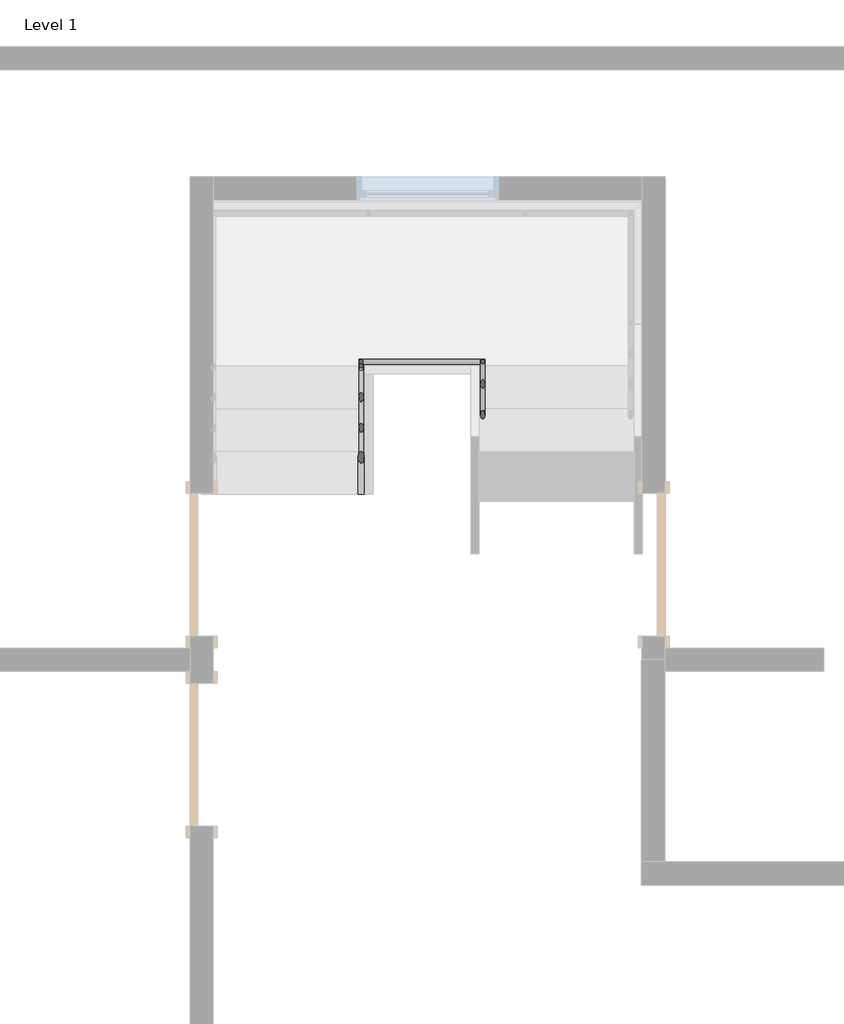
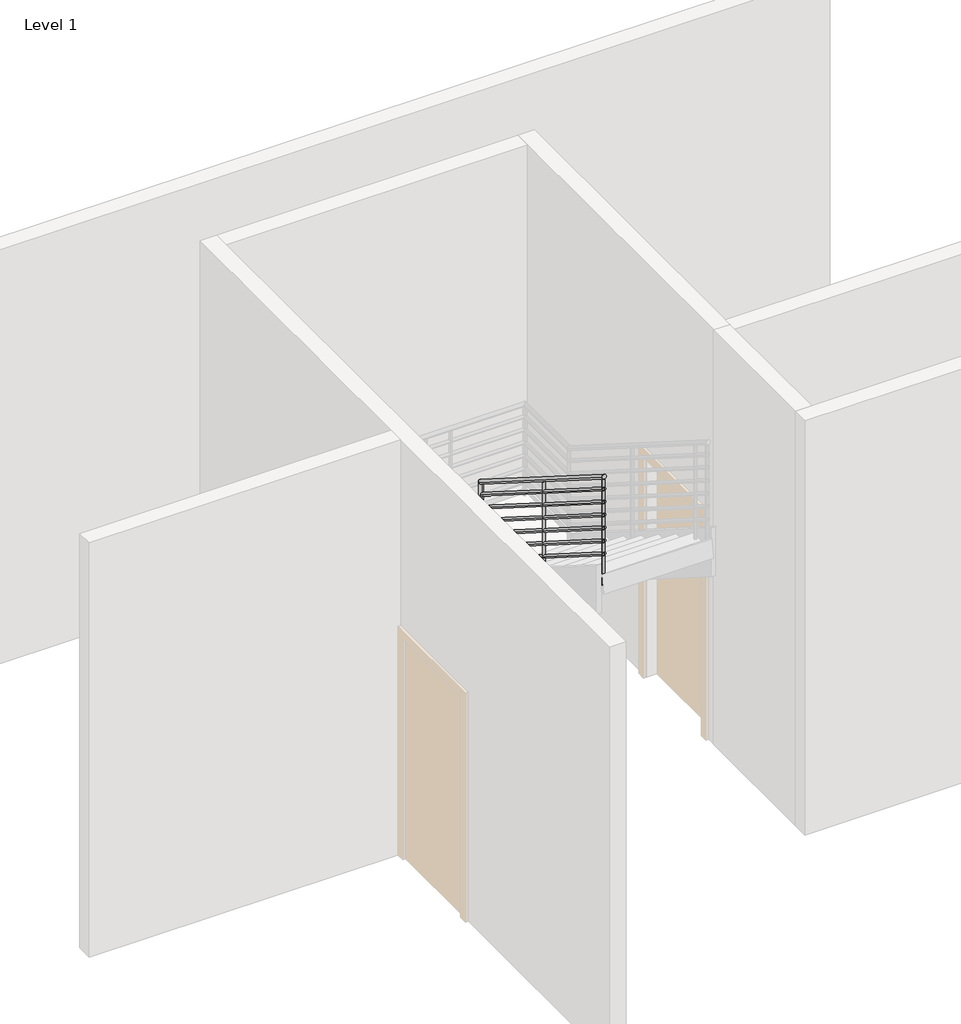
# One storey, part 2 of 3: 1 railing.
"""IFC4 building model written with IfcOpenShell, lengths in millimetres."""

from ifc_helpers import new_model, si_unit, point, frame, frame_2d, origin, place, context, project, spatial, circle_curve, ellipse_curve, trimmed, segment, composite_curve, outline, extrude, element, save
from ifc_brep_helpers import plane_surface, cylinder_surface, advanced_brep

model = new_model("IFC4")

# Units and contexts
model_context = context("Model", 3, world=origin())
ifc_project = project(units=[si_unit("LENGTHUNIT", "METRE", prefix="MILLI")], contexts=[model_context])

# Site, building, storey
site = spatial("IfcSite", under=ifc_project)
building = spatial("IfcBuilding", under=site)
storey = spatial("IfcBuildingStorey", under=building, Name="Level 1", Elevation=0.0)

# Railing
placement = place(None, origin())
element("IfcRailing", 1, ObjectType="900mm Pipe", at=placement, inside=storey, context=model_context, shape_type="SolidModel", body=[
    advanced_brep(
    [(-9602.5247141, 8997.57664, 1050.2491997), (-9642.5247141, 8997.57664, 1050.2491997), (-9602.5247141, 9841.7631282, 1584.1220776), (-9642.5247141, 9875.5699774, 1605.5019032)],
    [
        (0, 1, ellipse_curve(frame((-9622.5247141, 8997.57664, 1050.2491997), z_axis=(0.0, -1.0, 0.0), x_axis=(0.0, 0.0, -1.0)), 23.6638438, 20.0)),
        (1, 0, ellipse_curve(frame((-9622.5247141, 8997.57664, 1050.2491997), z_axis=(0.0, -1.0, 0.0), x_axis=(0.0, 0.0, -1.0)), 23.6638438, 20.0)),
        (2, 3, ellipse_curve(frame((-9622.5247141, 9858.6665528, 1594.8119904), z_axis=(0.7071067811865501, 0.597626308985335, 0.37794549184844306), x_axis=(0.7071067811865452, -0.5976263089853413, -0.3779454918484418)), 28.2842712, 20.0)),
        (3, 2, ellipse_curve(frame((-9622.5247141, 9858.6665528, 1594.8119904), z_axis=(0.7071067811865501, 0.597626308985335, 0.37794549184844306), x_axis=(0.7071067811865452, -0.5976263089853413, -0.3779454918484418)), 28.2842712, 20.0)),
        (0, 2),
        (3, 1),
    ],
    [
        plane_surface(frame((-9622.5247141, 8997.57664, 1073.9130435), z_axis=(0.0, -1.0, 0.0), x_axis=(0.0, 0.0, 1.0))),
        plane_surface(frame((-9622.5247141, 9847.97664, 1611.715415), z_axis=(0.7071067811865501, 0.597626308985335, 0.37794549184844306), x_axis=(0.707106781186545, -0.5976263089853392, -0.3779454918484457))),
        cylinder_surface(frame((-9622.5247141, 9008.2665528, 1057.0096189), z_axis=(0.0, -0.8451712313980392, -0.5344956404098373), x_axis=(-1.0, 0.0, 0.0)), 20.0),
    ],
    [
        (0, [[1, 2]]),
        (1, [[3, 4]]),
        (2, [[-1, 5, -4, 6]]),
        (2, [[-2, -6, -3, -5]]),
    ],
),
    advanced_brep(
    [(-9594.9313766, 9827.97664, 1575.6521739), (-9628.7382259, 9867.97664, 1575.6521739), (-8842.1141631, 9827.97664, 1575.6521739), (-8842.1141631, 9867.97664, 1575.6521739)],
    [
        (0, 1, ellipse_curve(frame((-9611.8348013, 9847.97664, 1575.6521739), z_axis=(-0.7071067811865501, -0.597626308985335, -0.37794549184844306), x_axis=(-0.7071067811865447, 0.5976263089853416, 0.377945491848442)), 28.2842712, 20.0)),
        (1, 0, ellipse_curve(frame((-9611.8348013, 9847.97664, 1575.6521739), z_axis=(-0.7071067811865501, -0.597626308985335, -0.37794549184844306), x_axis=(-0.7071067811865447, 0.5976263089853416, 0.377945491848442)), 28.2842712, 20.0)),
        (2, 3, ellipse_curve(frame((-8842.1141631, 9847.97664, 1575.6521739), z_axis=(0.7071067811865476, 0.0, 0.7071067811865476), x_axis=(-0.7071067811865474, 0.0, 0.7071067811865476)), 28.2842712, 20.0)),
        (3, 2, ellipse_curve(frame((-8842.1141631, 9847.97664, 1575.6521739), z_axis=(0.7071067811865476, 0.0, 0.7071067811865476), x_axis=(-0.7071067811865474, 0.0, 0.7071067811865476)), 28.2842712, 20.0)),
        (0, 2),
        (3, 1),
    ],
    [
        plane_surface(frame((-9622.5247141, 9847.97664, 1595.6521739), z_axis=(-0.7071067811865501, -0.597626308985335, -0.37794549184844306), x_axis=(0.707106781186545, -0.5976263089853392, -0.3779454918484457))),
        plane_surface(frame((-8862.1141631, 9847.97664, 1595.6521739), z_axis=(0.7071067811865476, 0.0, 0.7071067811865476), x_axis=(0.7071067811865476, 0.0, -0.7071067811865476))),
        cylinder_surface(frame((-9622.5247141, 9847.97664, 1575.6521739), z_axis=(-1.0, 0.0, 0.0), x_axis=(0.0, 1.0, 0.0)), 20.0),
    ],
    [
        (0, [[1, 2]]),
        (1, [[3, 4]]),
        (2, [[-1, 5, -4, 6]]),
        (2, [[-2, -6, -3, -5]]),
    ],
),
    advanced_brep(
    [(-8842.1141631, 9827.97664, 1575.6521739), (-8842.1141631, 9867.97664, 1575.6521739), (-8842.1141631, 9827.97664, 1718.82251), (-8842.1141631, 9867.97664, 1740.8537549)],
    [
        (0, 1, ellipse_curve(frame((-8842.1141631, 9847.97664, 1575.6521739), z_axis=(-0.7071067811865476, 0.0, -0.7071067811865476), x_axis=(0.7071067811865476, 0.0, -0.7071067811865474)), 28.2842712, 20.0)),
        (1, 0, ellipse_curve(frame((-8842.1141631, 9847.97664, 1575.6521739), z_axis=(-0.7071067811865476, 0.0, -0.7071067811865476), x_axis=(0.7071067811865476, 0.0, -0.7071067811865474)), 28.2842712, 20.0)),
        (2, 3, ellipse_curve(frame((-8842.1141631, 9847.97664, 1729.8381325), z_axis=(0.0, -0.4824439654458172, 0.8759268349610686), x_axis=(0.0, -0.8759268349610686, -0.48244396544581725)), 22.8329573, 20.0)),
        (3, 2, ellipse_curve(frame((-8842.1141631, 9847.97664, 1729.8381325), z_axis=(0.0, -0.4824439654458172, 0.8759268349610686), x_axis=(0.0, -0.8759268349610686, -0.48244396544581725)), 22.8329573, 20.0)),
        (0, 2),
        (3, 1),
    ],
    [
        plane_surface(frame((-8842.1141631, 9847.97664, 1575.6521739), z_axis=(-0.7071067811865476, 0.0, -0.7071067811865476), x_axis=(0.7071067811865476, 0.0, -0.7071067811865476))),
        plane_surface(frame((-8842.1141631, 9847.97664, 1729.8381325), z_axis=(0.0, -0.4824439654458172, 0.8759268349610686), x_axis=(1.0, 0.0, 0.0))),
        cylinder_surface(frame((-8842.1141631, 9847.97664, 1575.6521739), z_axis=(0.0, 0.0, -1.0), x_axis=(0.0, 1.0, 0.0)), 20.0),
    ],
    [
        (0, [[1, 2]]),
        (1, [[3, 4]]),
        (2, [[-1, 5, -4, 6]]),
        (2, [[-2, -6, -3, -5]]),
    ],
),
    advanced_brep(
    [(-8862.1141631, 9847.97664, 1729.8381325), (-8822.1141631, 9847.97664, 1729.8381325), (-8862.1141631, 7897.57664, 2963.2926779), (-8822.1141631, 7897.57664, 2963.2926779)],
    [
        (0, 1, ellipse_curve(frame((-8842.1141631, 9847.97664, 1729.8381325), z_axis=(0.0, 0.4824439654458172, -0.8759268349610686), x_axis=(0.0, 0.8759268349610685, 0.48244396544581725)), 22.8329573, 20.0)),
        (1, 0, ellipse_curve(frame((-8842.1141631, 9847.97664, 1729.8381325), z_axis=(0.0, 0.4824439654458172, -0.8759268349610686), x_axis=(0.0, 0.8759268349610685, 0.48244396544581725)), 22.8329573, 20.0)),
        (2, 3, ellipse_curve(frame((-8842.1141631, 7897.57664, 2963.2926779), z_axis=(0.0, -1.0, 0.0), x_axis=(0.0, 0.0, -1.0)), 23.6638438, 20.0)),
        (3, 2, ellipse_curve(frame((-8842.1141631, 7897.57664, 2963.2926779), z_axis=(0.0, -1.0, 0.0), x_axis=(0.0, 0.0, -1.0)), 23.6638438, 20.0)),
        (0, 2),
        (3, 1),
    ],
    [
        plane_surface(frame((-8842.1141631, 9867.97664, 1740.8537549), z_axis=(0.0, 0.4824439654458172, -0.8759268349610686), x_axis=(1.0, 0.0, 0.0))),
        plane_surface(frame((-8842.1141631, 7897.57664, 2986.9565217), z_axis=(0.0, -1.0, 0.0), x_axis=(0.0, 0.0, -1.0))),
        cylinder_surface(frame((-8842.1141631, 9857.2867272, 1723.9503303), z_axis=(0.0, 0.8451712313980436, -0.5344956404098303), x_axis=(1.0, 0.0, 0.0)), 20.0),
    ],
    [
        (0, [[1, 2]]),
        (1, [[3, 4]]),
        (2, [[-1, 5, -4, 6]]),
        (2, [[-2, -6, -3, -5]]),
    ],
),
    advanced_brep(
    [(-9637.5247141, 8997.57664, 931.1651606), (-9607.5247141, 8997.57664, 931.1651606), (-9637.5247141, 9826.9217297, 1455.6521739), (-9607.5247141, 9826.9217297, 1455.6521739), (-9637.5247141, 9862.97664, 1455.6521739), (-9607.5247141, 9832.97664, 1455.6521739), (-8857.1141631, 9862.97664, 1455.6521739), (-8857.1141631, 9832.97664, 1455.6521739)],
    [
        (0, 1, ellipse_curve(frame((-9622.5247141, 8997.57664, 931.1651606), z_axis=(0.0, -1.0, 0.0), x_axis=(0.0, 0.0, -1.0)), 17.7478828, 15.0)),
        (1, 0, ellipse_curve(frame((-9622.5247141, 8997.57664, 931.1651606), z_axis=(0.0, -1.0, 0.0), x_axis=(0.0, 0.0, -1.0)), 17.7478828, 15.0)),
        (0, 2),
        (2, 3, ellipse_curve(frame((-9622.5247141, 9826.9217297, 1455.6521739), z_axis=(0.0, -0.9605132043335062, -0.27823440531497945), x_axis=(0.0, 0.27823440531497956, -0.9605132043335062)), 15.6166515, 15.0)),
        (3, 1),
        (3, 2, ellipse_curve(frame((-9622.5247141, 9826.9217297, 1455.6521739), z_axis=(0.0, -0.9605132043335062, -0.27823440531497945), x_axis=(0.0, 0.27823440531497956, -0.9605132043335062)), 15.6166515, 15.0)),
        (2, 4),
        (4, 5, ellipse_curve(frame((-9622.5247141, 9847.97664, 1455.6521739), z_axis=(-0.7071067811865506, -0.7071067811865445, 0.0), x_axis=(0.7071067811865445, -0.7071067811865505, 0.0)), 21.2132034, 15.0)),
        (5, 3),
        (5, 4, ellipse_curve(frame((-9622.5247141, 9847.97664, 1455.6521739), z_axis=(-0.7071067811865506, -0.7071067811865445, 0.0), x_axis=(0.7071067811865445, -0.7071067811865505, 0.0)), 21.2132034, 15.0)),
        (6, 7, circle_curve(frame((-8857.1141631, 9847.97664, 1455.6521739), z_axis=(1.0, 0.0, 0.0), x_axis=(0.0, -1.0, 0.0)), 15.0)),
        (7, 6, circle_curve(frame((-8857.1141631, 9847.97664, 1455.6521739), z_axis=(1.0, 0.0, 0.0), x_axis=(0.0, -1.0, 0.0)), 15.0)),
        (4, 6),
        (7, 5),
    ],
    [
        plane_surface(frame((-9622.5247141, 8997.57664, 948.9130435), z_axis=(0.0, -1.0, 0.0), x_axis=(0.0, 0.0, 1.0))),
        cylinder_surface(frame((-9622.5247141, 9005.5940746, 936.235475), z_axis=(0.0, -0.8451712313980396, -0.5344956404098367), x_axis=(1.0, 0.0, 0.0)), 15.0),
        cylinder_surface(frame((-9622.5247141, 9822.57664, 1455.6521739), z_axis=(0.0, -1.0, 0.0), x_axis=(1.0, 0.0, 0.0)), 15.0),
        plane_surface(frame((-8857.1141631, 9847.97664, 1470.6521739), z_axis=(1.0, 0.0, 0.0), x_axis=(0.0, 1.0, 0.0))),
        cylinder_surface(frame((-9622.5247141, 9847.97664, 1455.6521739), z_axis=(-1.0, 0.0, 0.0), x_axis=(0.0, -1.0, 0.0)), 15.0),
    ],
    [
        (0, [[1, 2]]),
        (1, [[-1, 3, 4, 5]]),
        (1, [[-2, -5, 6, -3]]),
        (2, [[-4, 7, 8, 9]]),
        (2, [[-6, -9, 10, -7]]),
        (3, [[11, 12]]),
        (4, [[-8, 13, -12, 14]]),
        (4, [[-10, -14, -11, -13]]),
    ],
),
    advanced_brep(
    [(-8827.1141631, 9862.97664, 1601.2679274), (-8857.1141631, 9862.97664, 1601.2679274), (-8827.1141631, 7897.57664, 2844.2086389), (-8857.1141631, 7897.57664, 2844.2086389)],
    [
        (0, 1, ellipse_curve(frame((-8842.1141631, 9862.97664, 1601.2679274), z_axis=(0.0, 1.0, 0.0), x_axis=(0.0, 0.0, -1.0)), 17.7478828, 15.0)),
        (1, 0, ellipse_curve(frame((-8842.1141631, 9862.97664, 1601.2679274), z_axis=(0.0, 1.0, 0.0), x_axis=(0.0, 0.0, -1.0)), 17.7478828, 15.0)),
        (2, 3, ellipse_curve(frame((-8842.1141631, 7897.57664, 2844.2086389), z_axis=(0.0, -1.0, 0.0), x_axis=(0.0, 0.0, -1.0)), 17.7478828, 15.0)),
        (3, 2, ellipse_curve(frame((-8842.1141631, 7897.57664, 2844.2086389), z_axis=(0.0, -1.0, 0.0), x_axis=(0.0, 0.0, -1.0)), 17.7478828, 15.0)),
        (0, 2),
        (3, 1),
    ],
    [
        plane_surface(frame((-8842.1141631, 9862.97664, 1619.0158103), z_axis=(0.0, 1.0, 0.0), x_axis=(0.0, 0.0, -1.0))),
        plane_surface(frame((-8842.1141631, 7897.57664, 2861.9565217), z_axis=(0.0, -1.0, 0.0), x_axis=(0.0, 0.0, -1.0))),
        cylinder_surface(frame((-8842.1141631, 9854.9592054, 1606.3382418), z_axis=(0.0, 0.8451712313980437, -0.5344956404098302), x_axis=(-1.0, 0.0, 0.0)), 15.0),
    ],
    [
        (0, [[1, 2]]),
        (1, [[3, 4]]),
        (2, [[-1, 5, -4, 6]]),
        (2, [[-2, -6, -3, -5]]),
    ],
),
    advanced_brep(
    [(-9637.5247141, 8997.57664, 806.1651606), (-9607.5247141, 8997.57664, 806.1651606), (-9637.5247141, 9826.9217297, 1330.6521739), (-9607.5247141, 9826.9217297, 1330.6521739), (-9637.5247141, 9862.97664, 1330.6521739), (-9607.5247141, 9832.97664, 1330.6521739), (-8857.1141631, 9862.97664, 1330.6521739), (-8857.1141631, 9832.97664, 1330.6521739)],
    [
        (0, 1, ellipse_curve(frame((-9622.5247141, 8997.57664, 806.1651606), z_axis=(0.0, -1.0, 0.0), x_axis=(0.0, 0.0, -1.0)), 17.7478828, 15.0)),
        (1, 0, ellipse_curve(frame((-9622.5247141, 8997.57664, 806.1651606), z_axis=(0.0, -1.0, 0.0), x_axis=(0.0, 0.0, -1.0)), 17.7478828, 15.0)),
        (0, 2),
        (2, 3, ellipse_curve(frame((-9622.5247141, 9826.9217297, 1330.6521739), z_axis=(0.0, -0.9605132043335062, -0.27823440531497945), x_axis=(0.0, 0.27823440531497956, -0.9605132043335062)), 15.6166515, 15.0)),
        (3, 1),
        (3, 2, ellipse_curve(frame((-9622.5247141, 9826.9217297, 1330.6521739), z_axis=(0.0, -0.9605132043335062, -0.27823440531497945), x_axis=(0.0, 0.27823440531497956, -0.9605132043335062)), 15.6166515, 15.0)),
        (2, 4),
        (4, 5, ellipse_curve(frame((-9622.5247141, 9847.97664, 1330.6521739), z_axis=(-0.7071067811865506, -0.7071067811865445, 0.0), x_axis=(0.7071067811865445, -0.7071067811865505, 0.0)), 21.2132034, 15.0)),
        (5, 3),
        (5, 4, ellipse_curve(frame((-9622.5247141, 9847.97664, 1330.6521739), z_axis=(-0.7071067811865506, -0.7071067811865445, 0.0), x_axis=(0.7071067811865445, -0.7071067811865505, 0.0)), 21.2132034, 15.0)),
        (6, 7, circle_curve(frame((-8857.1141631, 9847.97664, 1330.6521739), z_axis=(1.0, 0.0, 0.0), x_axis=(0.0, -1.0, 0.0)), 15.0)),
        (7, 6, circle_curve(frame((-8857.1141631, 9847.97664, 1330.6521739), z_axis=(1.0, 0.0, 0.0), x_axis=(0.0, -1.0, 0.0)), 15.0)),
        (4, 6),
        (7, 5),
    ],
    [
        plane_surface(frame((-9622.5247141, 8997.57664, 823.9130435), z_axis=(0.0, -1.0, 0.0), x_axis=(0.0, 0.0, 1.0))),
        cylinder_surface(frame((-9622.5247141, 9005.5940746, 811.235475), z_axis=(0.0, -0.8451712313980396, -0.5344956404098367), x_axis=(1.0, 0.0, 0.0)), 15.0),
        cylinder_surface(frame((-9622.5247141, 9822.57664, 1330.6521739), z_axis=(0.0, -1.0, 0.0), x_axis=(1.0, 0.0, 0.0)), 15.0),
        plane_surface(frame((-8857.1141631, 9847.97664, 1345.6521739), z_axis=(1.0, 0.0, 0.0), x_axis=(0.0, 1.0, 0.0))),
        cylinder_surface(frame((-9622.5247141, 9847.97664, 1330.6521739), z_axis=(-1.0, 0.0, 0.0), x_axis=(0.0, -1.0, 0.0)), 15.0),
    ],
    [
        (0, [[1, 2]]),
        (1, [[-1, 3, 4, 5]]),
        (1, [[-2, -5, 6, -3]]),
        (2, [[-4, 7, 8, 9]]),
        (2, [[-6, -9, 10, -7]]),
        (3, [[11, 12]]),
        (4, [[-8, 13, -12, 14]]),
        (4, [[-10, -14, -11, -13]]),
    ],
),
    advanced_brep(
    [(-8827.1141631, 9862.97664, 1476.2679274), (-8857.1141631, 9862.97664, 1476.2679274), (-8827.1141631, 7897.57664, 2719.2086389), (-8857.1141631, 7897.57664, 2719.2086389)],
    [
        (0, 1, ellipse_curve(frame((-8842.1141631, 9862.97664, 1476.2679274), z_axis=(0.0, 1.0, 0.0), x_axis=(0.0, 0.0, -1.0)), 17.7478828, 15.0)),
        (1, 0, ellipse_curve(frame((-8842.1141631, 9862.97664, 1476.2679274), z_axis=(0.0, 1.0, 0.0), x_axis=(0.0, 0.0, -1.0)), 17.7478828, 15.0)),
        (2, 3, ellipse_curve(frame((-8842.1141631, 7897.57664, 2719.2086389), z_axis=(0.0, -1.0, 0.0), x_axis=(0.0, 0.0, -1.0)), 17.7478828, 15.0)),
        (3, 2, ellipse_curve(frame((-8842.1141631, 7897.57664, 2719.2086389), z_axis=(0.0, -1.0, 0.0), x_axis=(0.0, 0.0, -1.0)), 17.7478828, 15.0)),
        (0, 2),
        (3, 1),
    ],
    [
        plane_surface(frame((-8842.1141631, 9862.97664, 1494.0158103), z_axis=(0.0, 1.0, 0.0), x_axis=(0.0, 0.0, -1.0))),
        plane_surface(frame((-8842.1141631, 7897.57664, 2736.9565217), z_axis=(0.0, -1.0, 0.0), x_axis=(0.0, 0.0, -1.0))),
        cylinder_surface(frame((-8842.1141631, 9854.9592054, 1481.3382418), z_axis=(0.0, 0.8451712313980437, -0.5344956404098302), x_axis=(-1.0, 0.0, 0.0)), 15.0),
    ],
    [
        (0, [[1, 2]]),
        (1, [[3, 4]]),
        (2, [[-1, 5, -4, 6]]),
        (2, [[-2, -6, -3, -5]]),
    ],
),
    advanced_brep(
    [(-9637.5247141, 8997.57664, 681.1651606), (-9607.5247141, 8997.57664, 681.1651606), (-9637.5247141, 9826.9217297, 1205.6521739), (-9607.5247141, 9826.9217297, 1205.6521739), (-9637.5247141, 9862.97664, 1205.6521739), (-9607.5247141, 9832.97664, 1205.6521739), (-8857.1141631, 9862.97664, 1205.6521739), (-8857.1141631, 9832.97664, 1205.6521739)],
    [
        (0, 1, ellipse_curve(frame((-9622.5247141, 8997.57664, 681.1651606), z_axis=(0.0, -1.0, 0.0), x_axis=(0.0, 0.0, -1.0)), 17.7478828, 15.0)),
        (1, 0, ellipse_curve(frame((-9622.5247141, 8997.57664, 681.1651606), z_axis=(0.0, -1.0, 0.0), x_axis=(0.0, 0.0, -1.0)), 17.7478828, 15.0)),
        (0, 2),
        (2, 3, ellipse_curve(frame((-9622.5247141, 9826.9217297, 1205.6521739), z_axis=(0.0, -0.9605132043335062, -0.27823440531497945), x_axis=(0.0, 0.27823440531497956, -0.9605132043335062)), 15.6166515, 15.0)),
        (3, 1),
        (3, 2, ellipse_curve(frame((-9622.5247141, 9826.9217297, 1205.6521739), z_axis=(0.0, -0.9605132043335062, -0.27823440531497945), x_axis=(0.0, 0.27823440531497956, -0.9605132043335062)), 15.6166515, 15.0)),
        (2, 4),
        (4, 5, ellipse_curve(frame((-9622.5247141, 9847.97664, 1205.6521739), z_axis=(-0.7071067811865506, -0.7071067811865445, 0.0), x_axis=(0.7071067811865445, -0.7071067811865505, 0.0)), 21.2132034, 15.0)),
        (5, 3),
        (5, 4, ellipse_curve(frame((-9622.5247141, 9847.97664, 1205.6521739), z_axis=(-0.7071067811865506, -0.7071067811865445, 0.0), x_axis=(0.7071067811865445, -0.7071067811865505, 0.0)), 21.2132034, 15.0)),
        (6, 7, circle_curve(frame((-8857.1141631, 9847.97664, 1205.6521739), z_axis=(1.0, 0.0, 0.0), x_axis=(0.0, -1.0, 0.0)), 15.0)),
        (7, 6, circle_curve(frame((-8857.1141631, 9847.97664, 1205.6521739), z_axis=(1.0, 0.0, 0.0), x_axis=(0.0, -1.0, 0.0)), 15.0)),
        (4, 6),
        (7, 5),
    ],
    [
        plane_surface(frame((-9622.5247141, 8997.57664, 698.9130435), z_axis=(0.0, -1.0, 0.0), x_axis=(0.0, 0.0, 1.0))),
        cylinder_surface(frame((-9622.5247141, 9005.5940746, 686.235475), z_axis=(0.0, -0.8451712313980396, -0.5344956404098367), x_axis=(1.0, 0.0, 0.0)), 15.0),
        cylinder_surface(frame((-9622.5247141, 9822.57664, 1205.6521739), z_axis=(0.0, -1.0, 0.0), x_axis=(1.0, 0.0, 0.0)), 15.0),
        plane_surface(frame((-8857.1141631, 9847.97664, 1220.6521739), z_axis=(1.0, 0.0, 0.0), x_axis=(0.0, 1.0, 0.0))),
        cylinder_surface(frame((-9622.5247141, 9847.97664, 1205.6521739), z_axis=(-1.0, 0.0, 0.0), x_axis=(0.0, -1.0, 0.0)), 15.0),
    ],
    [
        (0, [[1, 2]]),
        (1, [[-1, 3, 4, 5]]),
        (1, [[-2, -5, 6, -3]]),
        (2, [[-4, 7, 8, 9]]),
        (2, [[-6, -9, 10, -7]]),
        (3, [[11, 12]]),
        (4, [[-8, 13, -12, 14]]),
        (4, [[-10, -14, -11, -13]]),
    ],
),
    advanced_brep(
    [(-8827.1141631, 9862.97664, 1351.2679274), (-8857.1141631, 9862.97664, 1351.2679274), (-8827.1141631, 7897.57664, 2594.2086389), (-8857.1141631, 7897.57664, 2594.2086389)],
    [
        (0, 1, ellipse_curve(frame((-8842.1141631, 9862.97664, 1351.2679274), z_axis=(0.0, 1.0, 0.0), x_axis=(0.0, 0.0, -1.0)), 17.7478828, 15.0)),
        (1, 0, ellipse_curve(frame((-8842.1141631, 9862.97664, 1351.2679274), z_axis=(0.0, 1.0, 0.0), x_axis=(0.0, 0.0, -1.0)), 17.7478828, 15.0)),
        (2, 3, ellipse_curve(frame((-8842.1141631, 7897.57664, 2594.2086389), z_axis=(0.0, -1.0, 0.0), x_axis=(0.0, 0.0, -1.0)), 17.7478828, 15.0)),
        (3, 2, ellipse_curve(frame((-8842.1141631, 7897.57664, 2594.2086389), z_axis=(0.0, -1.0, 0.0), x_axis=(0.0, 0.0, -1.0)), 17.7478828, 15.0)),
        (0, 2),
        (3, 1),
    ],
    [
        plane_surface(frame((-8842.1141631, 9862.97664, 1369.0158103), z_axis=(0.0, 1.0, 0.0), x_axis=(0.0, 0.0, -1.0))),
        plane_surface(frame((-8842.1141631, 7897.57664, 2611.9565217), z_axis=(0.0, -1.0, 0.0), x_axis=(0.0, 0.0, -1.0))),
        cylinder_surface(frame((-8842.1141631, 9854.9592054, 1356.3382418), z_axis=(0.0, 0.8451712313980436, -0.5344956404098304), x_axis=(-1.0, 0.0, 0.0)), 15.0),
    ],
    [
        (0, [[1, 2]]),
        (1, [[3, 4]]),
        (2, [[-1, 5, -4, 6]]),
        (2, [[-2, -6, -3, -5]]),
    ],
),
    advanced_brep(
    [(-9637.5247141, 8997.57664, 556.1651606), (-9607.5247141, 8997.57664, 556.1651606), (-9637.5247141, 9826.9217297, 1080.6521739), (-9607.5247141, 9826.9217297, 1080.6521739), (-9637.5247141, 9862.97664, 1080.6521739), (-9607.5247141, 9832.97664, 1080.6521739), (-8857.1141631, 9862.97664, 1080.6521739), (-8857.1141631, 9832.97664, 1080.6521739)],
    [
        (0, 1, ellipse_curve(frame((-9622.5247141, 8997.57664, 556.1651606), z_axis=(0.0, -1.0, 0.0), x_axis=(0.0, 0.0, -1.0)), 17.7478828, 15.0)),
        (1, 0, ellipse_curve(frame((-9622.5247141, 8997.57664, 556.1651606), z_axis=(0.0, -1.0, 0.0), x_axis=(0.0, 0.0, -1.0)), 17.7478828, 15.0)),
        (0, 2),
        (2, 3, ellipse_curve(frame((-9622.5247141, 9826.9217297, 1080.6521739), z_axis=(0.0, -0.9605132043335062, -0.27823440531497945), x_axis=(0.0, 0.27823440531497956, -0.9605132043335062)), 15.6166515, 15.0)),
        (3, 1),
        (3, 2, ellipse_curve(frame((-9622.5247141, 9826.9217297, 1080.6521739), z_axis=(0.0, -0.9605132043335062, -0.27823440531497945), x_axis=(0.0, 0.27823440531497956, -0.9605132043335062)), 15.6166515, 15.0)),
        (2, 4),
        (4, 5, ellipse_curve(frame((-9622.5247141, 9847.97664, 1080.6521739), z_axis=(-0.7071067811865506, -0.7071067811865445, 0.0), x_axis=(0.7071067811865445, -0.7071067811865505, 0.0)), 21.2132034, 15.0)),
        (5, 3),
        (5, 4, ellipse_curve(frame((-9622.5247141, 9847.97664, 1080.6521739), z_axis=(-0.7071067811865506, -0.7071067811865445, 0.0), x_axis=(0.7071067811865445, -0.7071067811865505, 0.0)), 21.2132034, 15.0)),
        (6, 7, circle_curve(frame((-8857.1141631, 9847.97664, 1080.6521739), z_axis=(1.0, 0.0, 0.0), x_axis=(0.0, -1.0, 0.0)), 15.0)),
        (7, 6, circle_curve(frame((-8857.1141631, 9847.97664, 1080.6521739), z_axis=(1.0, 0.0, 0.0), x_axis=(0.0, -1.0, 0.0)), 15.0)),
        (4, 6),
        (7, 5),
    ],
    [
        plane_surface(frame((-9622.5247141, 8997.57664, 573.9130435), z_axis=(0.0, -1.0, 0.0), x_axis=(0.0, 0.0, 1.0))),
        cylinder_surface(frame((-9622.5247141, 9005.5940746, 561.235475), z_axis=(0.0, -0.8451712313980396, -0.5344956404098367), x_axis=(1.0, 0.0, 0.0)), 15.0),
        cylinder_surface(frame((-9622.5247141, 9822.57664, 1080.6521739), z_axis=(0.0, -1.0, 0.0), x_axis=(1.0, 0.0, 0.0)), 15.0),
        plane_surface(frame((-8857.1141631, 9847.97664, 1095.6521739), z_axis=(1.0, 0.0, 0.0), x_axis=(0.0, 1.0, 0.0))),
        cylinder_surface(frame((-9622.5247141, 9847.97664, 1080.6521739), z_axis=(-1.0, 0.0, 0.0), x_axis=(0.0, -1.0, 0.0)), 15.0),
    ],
    [
        (0, [[1, 2]]),
        (1, [[-1, 3, 4, 5]]),
        (1, [[-2, -5, 6, -3]]),
        (2, [[-4, 7, 8, 9]]),
        (2, [[-6, -9, 10, -7]]),
        (3, [[11, 12]]),
        (4, [[-8, 13, -12, 14]]),
        (4, [[-10, -14, -11, -13]]),
    ],
),
    advanced_brep(
    [(-8827.1141631, 9862.97664, 1226.2679274), (-8857.1141631, 9862.97664, 1226.2679274), (-8827.1141631, 7897.57664, 2469.2086389), (-8857.1141631, 7897.57664, 2469.2086389)],
    [
        (0, 1, ellipse_curve(frame((-8842.1141631, 9862.97664, 1226.2679274), z_axis=(0.0, 1.0, 0.0), x_axis=(0.0, 0.0, -1.0)), 17.7478828, 15.0)),
        (1, 0, ellipse_curve(frame((-8842.1141631, 9862.97664, 1226.2679274), z_axis=(0.0, 1.0, 0.0), x_axis=(0.0, 0.0, -1.0)), 17.7478828, 15.0)),
        (2, 3, ellipse_curve(frame((-8842.1141631, 7897.57664, 2469.2086389), z_axis=(0.0, -1.0, 0.0), x_axis=(0.0, 0.0, -1.0)), 17.7478828, 15.0)),
        (3, 2, ellipse_curve(frame((-8842.1141631, 7897.57664, 2469.2086389), z_axis=(0.0, -1.0, 0.0), x_axis=(0.0, 0.0, -1.0)), 17.7478828, 15.0)),
        (0, 2),
        (3, 1),
    ],
    [
        plane_surface(frame((-8842.1141631, 9862.97664, 1244.0158103), z_axis=(0.0, 1.0, 0.0), x_axis=(0.0, 0.0, -1.0))),
        plane_surface(frame((-8842.1141631, 7897.57664, 2486.9565217), z_axis=(0.0, -1.0, 0.0), x_axis=(0.0, 0.0, -1.0))),
        cylinder_surface(frame((-8842.1141631, 9854.9592054, 1231.3382418), z_axis=(0.0, 0.8451712313980437, -0.5344956404098302), x_axis=(-1.0, 0.0, 0.0)), 15.0),
    ],
    [
        (0, [[1, 2]]),
        (1, [[3, 4]]),
        (2, [[-1, 5, -4, 6]]),
        (2, [[-2, -6, -3, -5]]),
    ],
),
    advanced_brep(
    [(-9637.5247141, 8997.57664, 431.1651606), (-9607.5247141, 8997.57664, 431.1651606), (-9637.5247141, 9826.9217297, 955.6521739), (-9607.5247141, 9826.9217297, 955.6521739), (-9637.5247141, 9862.97664, 955.6521739), (-9607.5247141, 9832.97664, 955.6521739), (-8857.1141631, 9862.97664, 955.6521739), (-8857.1141631, 9832.97664, 955.6521739)],
    [
        (0, 1, ellipse_curve(frame((-9622.5247141, 8997.57664, 431.1651606), z_axis=(0.0, -1.0, 0.0), x_axis=(0.0, 0.0, -1.0)), 17.7478828, 15.0)),
        (1, 0, ellipse_curve(frame((-9622.5247141, 8997.57664, 431.1651606), z_axis=(0.0, -1.0, 0.0), x_axis=(0.0, 0.0, -1.0)), 17.7478828, 15.0)),
        (0, 2),
        (2, 3, ellipse_curve(frame((-9622.5247141, 9826.9217297, 955.6521739), z_axis=(0.0, -0.9605132043335062, -0.27823440531497945), x_axis=(0.0, 0.27823440531497956, -0.9605132043335062)), 15.6166515, 15.0)),
        (3, 1),
        (3, 2, ellipse_curve(frame((-9622.5247141, 9826.9217297, 955.6521739), z_axis=(0.0, -0.9605132043335062, -0.27823440531497945), x_axis=(0.0, 0.27823440531497956, -0.9605132043335062)), 15.6166515, 15.0)),
        (2, 4),
        (4, 5, ellipse_curve(frame((-9622.5247141, 9847.97664, 955.6521739), z_axis=(-0.7071067811865506, -0.7071067811865445, 0.0), x_axis=(0.7071067811865445, -0.7071067811865505, 0.0)), 21.2132034, 15.0)),
        (5, 3),
        (5, 4, ellipse_curve(frame((-9622.5247141, 9847.97664, 955.6521739), z_axis=(-0.7071067811865506, -0.7071067811865445, 0.0), x_axis=(0.7071067811865445, -0.7071067811865505, 0.0)), 21.2132034, 15.0)),
        (6, 7, circle_curve(frame((-8857.1141631, 9847.97664, 955.6521739), z_axis=(1.0, 0.0, 0.0), x_axis=(0.0, -1.0, 0.0)), 15.0)),
        (7, 6, circle_curve(frame((-8857.1141631, 9847.97664, 955.6521739), z_axis=(1.0, 0.0, 0.0), x_axis=(0.0, -1.0, 0.0)), 15.0)),
        (4, 6),
        (7, 5),
    ],
    [
        plane_surface(frame((-9622.5247141, 8997.57664, 448.9130435), z_axis=(0.0, -1.0, 0.0), x_axis=(0.0, 0.0, 1.0))),
        cylinder_surface(frame((-9622.5247141, 9005.5940746, 436.235475), z_axis=(0.0, -0.8451712313980396, -0.5344956404098367), x_axis=(1.0, 0.0, 0.0)), 15.0),
        cylinder_surface(frame((-9622.5247141, 9822.57664, 955.6521739), z_axis=(0.0, -1.0, 0.0), x_axis=(1.0, 0.0, 0.0)), 15.0),
        plane_surface(frame((-8857.1141631, 9847.97664, 970.6521739), z_axis=(1.0, 0.0, 0.0), x_axis=(0.0, 1.0, 0.0))),
        cylinder_surface(frame((-9622.5247141, 9847.97664, 955.6521739), z_axis=(-1.0, 0.0, 0.0), x_axis=(0.0, -1.0, 0.0)), 15.0),
    ],
    [
        (0, [[1, 2]]),
        (1, [[-1, 3, 4, 5]]),
        (1, [[-2, -5, 6, -3]]),
        (2, [[-4, 7, 8, 9]]),
        (2, [[-6, -9, 10, -7]]),
        (3, [[11, 12]]),
        (4, [[-8, 13, -12, 14]]),
        (4, [[-10, -14, -11, -13]]),
    ],
),
    advanced_brep(
    [(-8827.1141631, 9862.97664, 1101.2679274), (-8857.1141631, 9862.97664, 1101.2679274), (-8827.1141631, 7897.57664, 2344.2086389), (-8857.1141631, 7897.57664, 2344.2086389)],
    [
        (0, 1, ellipse_curve(frame((-8842.1141631, 9862.97664, 1101.2679274), z_axis=(0.0, 1.0, 0.0), x_axis=(0.0, 0.0, -1.0)), 17.7478828, 15.0)),
        (1, 0, ellipse_curve(frame((-8842.1141631, 9862.97664, 1101.2679274), z_axis=(0.0, 1.0, 0.0), x_axis=(0.0, 0.0, -1.0)), 17.7478828, 15.0)),
        (2, 3, ellipse_curve(frame((-8842.1141631, 7897.57664, 2344.2086389), z_axis=(0.0, -1.0, 0.0), x_axis=(0.0, 0.0, -1.0)), 17.7478828, 15.0)),
        (3, 2, ellipse_curve(frame((-8842.1141631, 7897.57664, 2344.2086389), z_axis=(0.0, -1.0, 0.0), x_axis=(0.0, 0.0, -1.0)), 17.7478828, 15.0)),
        (0, 2),
        (3, 1),
    ],
    [
        plane_surface(frame((-8842.1141631, 9862.97664, 1119.0158103), z_axis=(0.0, 1.0, 0.0), x_axis=(0.0, 0.0, -1.0))),
        plane_surface(frame((-8842.1141631, 7897.57664, 2361.9565217), z_axis=(0.0, -1.0, 0.0), x_axis=(0.0, 0.0, -1.0))),
        cylinder_surface(frame((-8842.1141631, 9854.9592054, 1106.3382418), z_axis=(0.0, 0.8451712313980437, -0.5344956404098302), x_axis=(-1.0, 0.0, 0.0)), 15.0),
    ],
    [
        (0, [[1, 2]]),
        (1, [[3, 4]]),
        (2, [[-1, 5, -4, 6]]),
        (2, [[-2, -6, -3, -5]]),
    ],
),
    advanced_brep(
    [(-9637.5247141, 8997.57664, 306.1651606), (-9607.5247141, 8997.57664, 306.1651606), (-9637.5247141, 9826.9217297, 830.6521739), (-9607.5247141, 9826.9217297, 830.6521739), (-9637.5247141, 9862.97664, 830.6521739), (-9607.5247141, 9832.97664, 830.6521739), (-8857.1141631, 9862.97664, 830.6521739), (-8857.1141631, 9832.97664, 830.6521739)],
    [
        (0, 1, ellipse_curve(frame((-9622.5247141, 8997.57664, 306.1651606), z_axis=(0.0, -1.0, 0.0), x_axis=(0.0, 0.0, -1.0)), 17.7478828, 15.0)),
        (1, 0, ellipse_curve(frame((-9622.5247141, 8997.57664, 306.1651606), z_axis=(0.0, -1.0, 0.0), x_axis=(0.0, 0.0, -1.0)), 17.7478828, 15.0)),
        (0, 2),
        (2, 3, ellipse_curve(frame((-9622.5247141, 9826.9217297, 830.6521739), z_axis=(0.0, -0.9605132043335062, -0.27823440531497945), x_axis=(0.0, 0.27823440531497956, -0.9605132043335062)), 15.6166515, 15.0)),
        (3, 1),
        (3, 2, ellipse_curve(frame((-9622.5247141, 9826.9217297, 830.6521739), z_axis=(0.0, -0.9605132043335062, -0.27823440531497945), x_axis=(0.0, 0.27823440531497956, -0.9605132043335062)), 15.6166515, 15.0)),
        (2, 4),
        (4, 5, ellipse_curve(frame((-9622.5247141, 9847.97664, 830.6521739), z_axis=(-0.7071067811865506, -0.7071067811865445, 0.0), x_axis=(0.7071067811865445, -0.7071067811865505, 0.0)), 21.2132034, 15.0)),
        (5, 3),
        (5, 4, ellipse_curve(frame((-9622.5247141, 9847.97664, 830.6521739), z_axis=(-0.7071067811865506, -0.7071067811865445, 0.0), x_axis=(0.7071067811865445, -0.7071067811865505, 0.0)), 21.2132034, 15.0)),
        (6, 7, circle_curve(frame((-8857.1141631, 9847.97664, 830.6521739), z_axis=(1.0, 0.0, 0.0), x_axis=(0.0, -1.0, 0.0)), 15.0)),
        (7, 6, circle_curve(frame((-8857.1141631, 9847.97664, 830.6521739), z_axis=(1.0, 0.0, 0.0), x_axis=(0.0, -1.0, 0.0)), 15.0)),
        (4, 6),
        (7, 5),
    ],
    [
        plane_surface(frame((-9622.5247141, 8997.57664, 323.9130435), z_axis=(0.0, -1.0, 0.0), x_axis=(0.0, 0.0, 1.0))),
        cylinder_surface(frame((-9622.5247141, 9005.5940746, 311.235475), z_axis=(0.0, -0.8451712313980396, -0.5344956404098367), x_axis=(1.0, 0.0, 0.0)), 15.0),
        cylinder_surface(frame((-9622.5247141, 9822.57664, 830.6521739), z_axis=(0.0, -1.0, 0.0), x_axis=(1.0, 0.0, 0.0)), 15.0),
        plane_surface(frame((-8857.1141631, 9847.97664, 845.6521739), z_axis=(1.0, 0.0, 0.0), x_axis=(0.0, 1.0, 0.0))),
        cylinder_surface(frame((-9622.5247141, 9847.97664, 830.6521739), z_axis=(-1.0, 0.0, 0.0), x_axis=(0.0, -1.0, 0.0)), 15.0),
    ],
    [
        (0, [[1, 2]]),
        (1, [[-1, 3, 4, 5]]),
        (1, [[-2, -5, 6, -3]]),
        (2, [[-4, 7, 8, 9]]),
        (2, [[-6, -9, 10, -7]]),
        (3, [[11, 12]]),
        (4, [[-8, 13, -12, 14]]),
        (4, [[-10, -14, -11, -13]]),
    ],
),
    advanced_brep(
    [(-8827.1141631, 9862.97664, 976.2679274), (-8857.1141631, 9862.97664, 976.2679274), (-8827.1141631, 7897.57664, 2219.2086389), (-8857.1141631, 7897.57664, 2219.2086389)],
    [
        (0, 1, ellipse_curve(frame((-8842.1141631, 9862.97664, 976.2679274), z_axis=(0.0, 1.0, 0.0), x_axis=(0.0, 0.0, -1.0)), 17.7478828, 15.0)),
        (1, 0, ellipse_curve(frame((-8842.1141631, 9862.97664, 976.2679274), z_axis=(0.0, 1.0, 0.0), x_axis=(0.0, 0.0, -1.0)), 17.7478828, 15.0)),
        (2, 3, ellipse_curve(frame((-8842.1141631, 7897.57664, 2219.2086389), z_axis=(0.0, -1.0, 0.0), x_axis=(0.0, 0.0, -1.0)), 17.7478828, 15.0)),
        (3, 2, ellipse_curve(frame((-8842.1141631, 7897.57664, 2219.2086389), z_axis=(0.0, -1.0, 0.0), x_axis=(0.0, 0.0, -1.0)), 17.7478828, 15.0)),
        (0, 2),
        (3, 1),
    ],
    [
        plane_surface(frame((-8842.1141631, 9862.97664, 994.0158103), z_axis=(0.0, 1.0, 0.0), x_axis=(0.0, 0.0, -1.0))),
        plane_surface(frame((-8842.1141631, 7897.57664, 2236.9565217), z_axis=(0.0, -1.0, 0.0), x_axis=(0.0, 0.0, -1.0))),
        cylinder_surface(frame((-8842.1141631, 9854.9592054, 981.3382418), z_axis=(0.0, 0.8451712313980437, -0.5344956404098302), x_axis=(-1.0, 0.0, 0.0)), 15.0),
    ],
    [
        (0, [[1, 2]]),
        (1, [[3, 4]]),
        (2, [[-1, 5, -4, 6]]),
        (2, [[-2, -6, -3, -5]]),
    ],
),
    advanced_brep(
    [(-8854.6141631, 8847.97664, 2338.5853559), (-8854.6141631, 8847.97664, 1391.3043478), (-8829.6141631, 8847.97664, 1391.3043478), (-8829.6141631, 8847.97664, 2338.5853559)],
    [
        (0, 1),
        (1, 2, circle_curve(frame((-8842.1141631, 8847.97664, 1391.3043478), z_axis=(0.0, 0.0, 1.0), x_axis=(1.0, 0.0, 0.0)), 12.5)),
        (2, 3),
        (3, 0, ellipse_curve(frame((-8842.1141631, 8847.97664, 2338.5853559), z_axis=(0.0, -0.5344956404098286, -0.8451712313980447), x_axis=(0.0, -0.8451712313980447, 0.5344956404098286)), 14.7899024, 12.5)),
        (0, 3, ellipse_curve(frame((-8842.1141631, 8847.97664, 2338.5853559), z_axis=(0.0, -0.5344956404098286, -0.8451712313980447), x_axis=(0.0, -0.8451712313980447, 0.5344956404098286)), 14.7899024, 12.5)),
        (2, 1, circle_curve(frame((-8842.1141631, 8847.97664, 1391.3043478), z_axis=(0.0, 0.0, 1.0), x_axis=(1.0, 0.0, 0.0)), 12.5)),
    ],
    [
        cylinder_surface(frame((-8842.1141631, 8847.97664, 1291.3043478), z_axis=(0.0, 0.0, 1.0), x_axis=(1.0, 0.0, 0.0)), 12.5),
        plane_surface(frame((-8817.1141631, 8822.97664, 2354.3956326), z_axis=(0.0, 0.5344956404098286, 0.8451712313980447), x_axis=(-1.0, 0.0, 0.0))),
        plane_surface(frame((-8817.1141631, 8872.97664, 1391.3043478), z_axis=(0.0, 0.0, -1.0), x_axis=(-1.0, 0.0, 0.0))),
    ],
    [
        (0, [[1, 2, 3, 4]]),
        (0, [[-1, 5, -3, 6]]),
        (1, [[-4, -5]]),
        (2, [[-2, -6]]),
    ],
),
    extrude(outline(composite_curve([segment(trimmed(circle_curve(frame_2d((-8842.1141631, 9847.97664)), 12.5), [point((-8829.6141631, 9847.97664))], [point((-8854.6141631, 9847.97664))], False, "CARTESIAN"), True, "CONTINUOUS"), segment(trimmed(circle_curve(frame_2d((-8842.1141631, 9847.97664)), 12.5), [point((-8854.6141631, 9847.97664))], [point((-8829.6141631, 9847.97664))], False, "CARTESIAN"), True, "CONTINUOUS")], self_intersect=False)), frame((0.0, 0.0, 695.6521739), z_axis=(0.0, 0.0, 1.0), x_axis=(1.0, 0.0, 0.0)), (0.0, 0.0, 1.0), 860.0),
    advanced_brep(
    [(-9610.0247141, 9847.97664, 1564.3877274), (-9610.0247141, 9847.97664, 695.6521739), (-9635.0247141, 9847.97664, 695.6521739), (-9635.0247141, 9847.97664, 1564.3877274)],
    [
        (0, 1),
        (1, 2, circle_curve(frame((-9622.5247141, 9847.97664, 695.6521739), z_axis=(0.0, 0.0, 1.0), x_axis=(-1.0, 0.0, 0.0)), 12.5)),
        (2, 3),
        (3, 0, ellipse_curve(frame((-9622.5247141, 9847.97664, 1564.3877274), z_axis=(0.0, 0.5344956404098368, -0.8451712313980396), x_axis=(0.0, 0.8451712313980398, 0.5344956404098364)), 14.7899024, 12.5)),
        (0, 3, ellipse_curve(frame((-9622.5247141, 9847.97664, 1564.3877274), z_axis=(0.0, 0.5344956404098368, -0.8451712313980396), x_axis=(0.0, 0.8451712313980398, 0.5344956404098364)), 14.7899024, 12.5)),
        (2, 1, circle_curve(frame((-9622.5247141, 9847.97664, 695.6521739), z_axis=(0.0, 0.0, 1.0), x_axis=(-1.0, 0.0, 0.0)), 12.5)),
    ],
    [
        cylinder_surface(frame((-9622.5247141, 9847.97664, 595.6521739), z_axis=(0.0, 0.0, 1.0), x_axis=(-1.0, 0.0, 0.0)), 12.5),
        plane_surface(frame((-9647.5247141, 9872.97664, 1580.1980041), z_axis=(0.0, -0.5344956404098368, 0.8451712313980396), x_axis=(1.0, 0.0, 0.0))),
        plane_surface(frame((-9647.5247141, 9822.97664, 695.6521739), z_axis=(0.0, 0.0, -1.0), x_axis=(1.0, 0.0, 0.0))),
    ],
    [
        (0, [[1, 2, 3, 4]]),
        (0, [[-1, 5, -3, 6]]),
        (1, [[-4, -5]]),
        (2, [[-2, -6]]),
    ],
),
    advanced_brep(
    [(-9610.0247141, 9822.57664, 1548.3244863), (-9610.0247141, 9822.57664, 695.6521739), (-9635.0247141, 9822.57664, 695.6521739), (-9635.0247141, 9822.57664, 1548.3244863)],
    [
        (0, 1),
        (1, 2, circle_curve(frame((-9622.5247141, 9822.57664, 695.6521739), z_axis=(0.0, 0.0, 1.0), x_axis=(-1.0, 0.0, 0.0)), 12.5)),
        (2, 3),
        (3, 0, ellipse_curve(frame((-9622.5247141, 9822.57664, 1548.3244863), z_axis=(0.0, 0.5344956404098368, -0.8451712313980396), x_axis=(0.0, 0.8451712313980398, 0.5344956404098364)), 14.7899024, 12.5)),
        (0, 3, ellipse_curve(frame((-9622.5247141, 9822.57664, 1548.3244863), z_axis=(0.0, 0.5344956404098368, -0.8451712313980396), x_axis=(0.0, 0.8451712313980398, 0.5344956404098364)), 14.7899024, 12.5)),
        (2, 1, circle_curve(frame((-9622.5247141, 9822.57664, 695.6521739), z_axis=(0.0, 0.0, 1.0), x_axis=(-1.0, 0.0, 0.0)), 12.5)),
    ],
    [
        cylinder_surface(frame((-9622.5247141, 9822.57664, 595.6521739), z_axis=(0.0, 0.0, 1.0), x_axis=(-1.0, 0.0, 0.0)), 12.5),
        plane_surface(frame((-9647.5247141, 9847.57664, 1564.134763), z_axis=(0.0, -0.5344956404098368, 0.8451712313980396), x_axis=(1.0, 0.0, 0.0))),
        plane_surface(frame((-9647.5247141, 9797.57664, 695.6521739), z_axis=(0.0, 0.0, -1.0), x_axis=(1.0, 0.0, 0.0))),
    ],
    [
        (0, [[1, 2, 3, 4]]),
        (0, [[-1, 5, -3, 6]]),
        (1, [[-4, -5]]),
        (2, [[-2, -6]]),
    ],
),
    advanced_brep(
    [(-8854.6141631, 7910.07664, 2931.7236958), (-8854.6141631, 7910.07664, 1913.0434783), (-8829.6141631, 7910.07664, 1913.0434783), (-8829.6141631, 7910.07664, 2931.7236958)],
    [
        (0, 1),
        (1, 2, circle_curve(frame((-8842.1141631, 7910.07664, 1913.0434783), z_axis=(0.0, 0.0, 1.0), x_axis=(1.0, 0.0, 0.0)), 12.5)),
        (2, 3),
        (3, 0, ellipse_curve(frame((-8842.1141631, 7910.07664, 2931.7236958), z_axis=(0.0, -0.5344956404098302, -0.8451712313980437), x_axis=(0.0, -0.8451712313980437, 0.53449564040983)), 14.7899024, 12.5)),
        (0, 3, ellipse_curve(frame((-8842.1141631, 7910.07664, 2931.7236958), z_axis=(0.0, -0.5344956404098302, -0.8451712313980437), x_axis=(0.0, -0.8451712313980437, 0.53449564040983)), 14.7899024, 12.5)),
        (2, 1, circle_curve(frame((-8842.1141631, 7910.07664, 1913.0434783), z_axis=(0.0, 0.0, 1.0), x_axis=(1.0, 0.0, 0.0)), 12.5)),
    ],
    [
        cylinder_surface(frame((-8842.1141631, 7910.07664, 1813.0434783), z_axis=(0.0, 0.0, 1.0), x_axis=(1.0, 0.0, 0.0)), 12.5),
        plane_surface(frame((-8817.1141631, 7885.07664, 2947.5339725), z_axis=(0.0, 0.5344956404098302, 0.8451712313980437), x_axis=(-1.0, 0.0, 0.0))),
        plane_surface(frame((-8817.1141631, 7935.07664, 1913.0434783), z_axis=(0.0, 0.0, -1.0), x_axis=(-1.0, 0.0, 0.0))),
    ],
    [
        (0, [[1, 2, 3, 4]]),
        (0, [[-1, 5, -3, 6]]),
        (1, [[-4, -5]]),
        (2, [[-2, -6]]),
    ],
),
    advanced_brep(
    [(-9610.0247141, 9010.07664, 1034.4904942), (-9610.0247141, 9010.07664, 173.9130435), (-9635.0247141, 9010.07664, 173.9130435), (-9635.0247141, 9010.07664, 1034.4904942)],
    [
        (0, 1),
        (1, 2, circle_curve(frame((-9622.5247141, 9010.07664, 173.9130435), z_axis=(0.0, 0.0, 1.0), x_axis=(-1.0, 0.0, 0.0)), 12.5)),
        (2, 3),
        (3, 0, ellipse_curve(frame((-9622.5247141, 9010.07664, 1034.4904942), z_axis=(0.0, 0.5344956404098368, -0.8451712313980396), x_axis=(0.0, 0.8451712313980398, 0.5344956404098364)), 14.7899024, 12.5)),
        (0, 3, ellipse_curve(frame((-9622.5247141, 9010.07664, 1034.4904942), z_axis=(0.0, 0.5344956404098368, -0.8451712313980396), x_axis=(0.0, 0.8451712313980398, 0.5344956404098364)), 14.7899024, 12.5)),
        (2, 1, circle_curve(frame((-9622.5247141, 9010.07664, 173.9130435), z_axis=(0.0, 0.0, 1.0), x_axis=(-1.0, 0.0, 0.0)), 12.5)),
    ],
    [
        cylinder_surface(frame((-9622.5247141, 9010.07664, 73.9130435), z_axis=(0.0, 0.0, 1.0), x_axis=(-1.0, 0.0, 0.0)), 12.5),
        plane_surface(frame((-9647.5247141, 9035.07664, 1050.3007709), z_axis=(0.0, -0.5344956404098368, 0.8451712313980396), x_axis=(1.0, 0.0, 0.0))),
        plane_surface(frame((-9647.5247141, 8985.07664, 173.9130435), z_axis=(0.0, 0.0, -1.0), x_axis=(1.0, 0.0, 0.0))),
    ],
    [
        (0, [[1, 2, 3, 4]]),
        (0, [[-1, 5, -3, 6]]),
        (1, [[-4, -5]]),
        (2, [[-2, -6]]),
    ],
),
])

save(model, "model.ifc")

# Revit data of these elements
# Type "900mm Pipe"
#   built-in parameter 1008612 = 0.019685 (stored number, unit not read)
#   built-in parameter 1008611 = 0.0984252 (stored number, unit not read)
#   built-in parameter 1008609 = 6.56168 (stored number, unit not read)
#   built-in parameter 1008604 = 0.19685 (stored number, unit not read)
#   built-in parameter 1008603 = 0.164042 (stored number, unit not read)
#   Railing Height = 900 mm
#   built-in parameter 1008630 = 2
#   built-in parameter 1008610 = 2
#   built-in parameter 1008605 = 1
#   built-in parameter 1008618 = M_Baluster - Round : 25mm
# Element 1 (IfcRailing, "900mm Pipe")
#   Phase Created = New Construction
